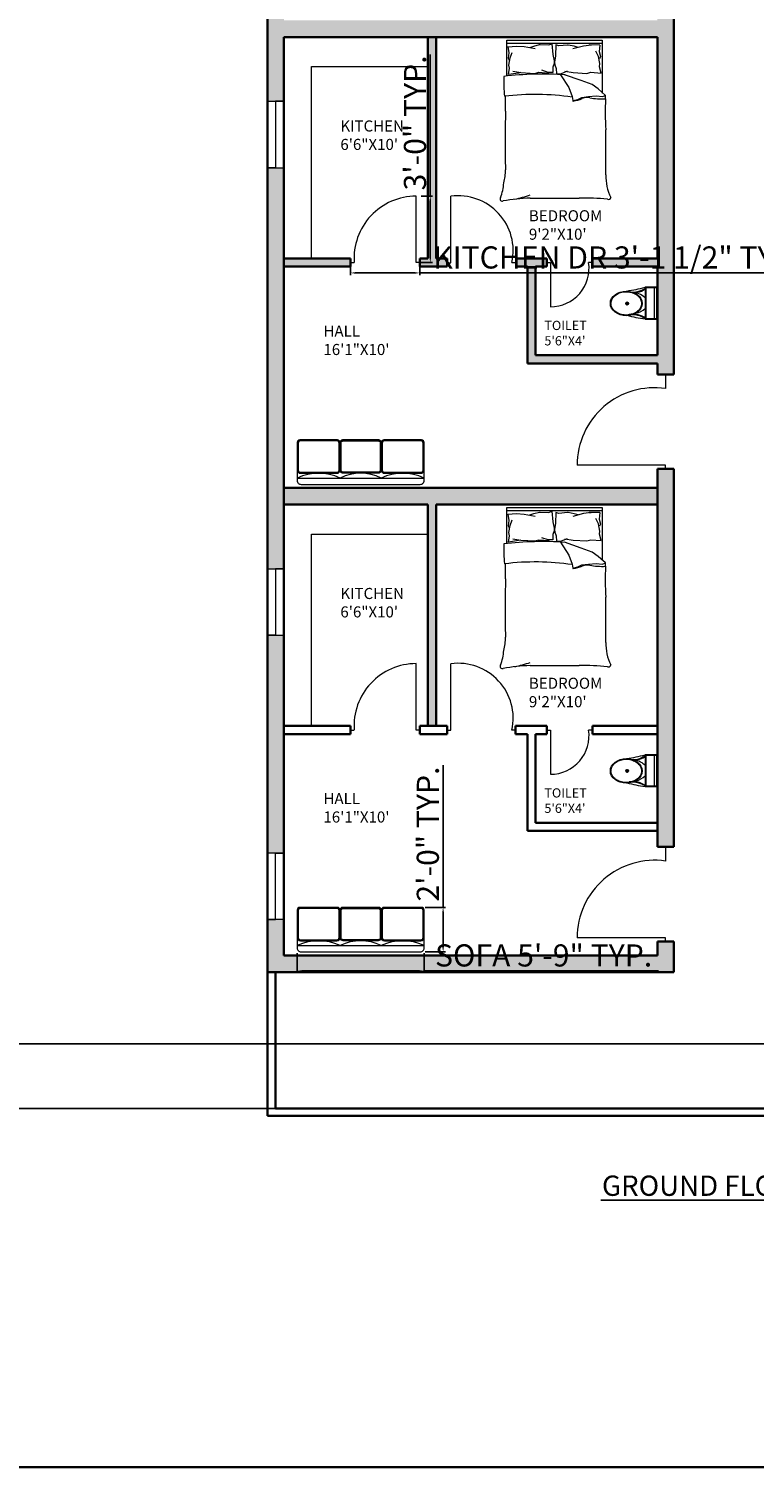
# Model space of a CAD drawing. Units: inches. Extents: x 1266 to 2869, y -408 to 3241.
# Tile 6 of 11: x 2023 to 2416, y 987 to 1767. Entities that reach past the tile are written whole.
import ezdxf

# ---------------------------------------------------------------- set-up
doc = ezdxf.new("R2010")
doc.units = ezdxf.units.IN
for name, color, linetype, lineweight in [('A-ANNO-DIMS', 2, 'Continuous', 18), ('A-ANNO-TITL', 7, 'Continuous', 25), ('A-ANNO-TTLB', 7, 'Continuous', 35), ('A-AREA-IDEN', 7, 'Continuous', 18), ('A-DOOR', 4, 'Continuous', 18), ('A-FLOR-CASE', 9, 'Continuous', 18), ('A-FLOR-FIXT', 9, 'Continuous', 18), ('A-FURN', 8, 'Continuous', 18), ('A-GLAZ', 4, 'Continuous', 18), ('A-WALL', 7, 'Continuous', 35), ('A-WALL-PATT', 251, 'Continuous', 13)]:
    doc.layers.add(name, color=color, linetype=linetype, lineweight=lineweight)
doc.styles.get("Standard").update_dxf_attribs({"font": 'arial.ttf'})
doc.dimstyles.new('ISO-25', dxfattribs={"dimtxt": 12, "dimasz": 2.5, "dimexe": 1.25, "dimexo": 0.625, "dimtad": 1, "dimdec": 0, "dimlunit": 3, "dimtxsty": 'Standard', "dimcen": 2.5, "dimadec": 0, "dimazin": 0, "dimtfac": 1, "dimtdec": 0, "dimtmove": 0, "dimatfit": 3, "dimfxl": 1, "dimarcsym": 0})

# ---------------------------------------------------------------- blocks, each defined once
blk = doc.blocks.new('A$C31115884')
for p, q in [((283, 498), (223, 498)), ((258, 466), (258, 523)), ((0, 200), (0, 0)), ((520, 200), (0, 200)), ((510, 54), (0, 54)), ((10, 190), (10, 10)), ((510, 190), (10, 190)), ((10, 10), (510, 10)), ((510, 10), (510, 190)), ((520, 0), (520, 200)), ((0, 0), (520, 0))]:
    blk.add_line(p, q)
blk.add_circle((256, 496), 23.6)
for centre, radius, start, end in [((2778, -205), 2807, 165.4549, 171.7133), ((3237, 905), 2807, 188.2867, 194.5451), ((-295, 403), 365, 324.2091, 9.3499), ((-295, 403), 375, 324.2091, 9.3499), ((384, 406), 293, 190.2774, 224.1564), ((139, 406), 293, 315.8436, 2.6563), ((806, 403), 375, 179.2036, 215.7909), ((806, 403), 365, 170.6501, 215.7909)]:
    blk.add_arc(centre, radius, start, end)
blk.add_ellipse((256, 510), major_axis=(0, -261), ratio=0.772727)
blk.add_open_spline([(256, 259), (263, 259), (270, 260), (288, 262), (299, 265), (320, 273), (330, 278), (350, 291), (360, 299), (378, 316), (386, 326), (402, 347), (409, 358), (421, 383), (427, 395), (436, 422), (440, 436), (445, 465), (447, 480), (448, 509), (448, 524), (445, 553), (443, 568), (436, 596), (432, 610), (422, 636), (416, 649), (402, 672), (395, 683), (379, 703), (370, 712), (351, 728), (341, 735), (321, 746), (310, 751), (289, 757), (278, 759), (256, 761), (245, 761), (223, 757), (212, 754), (191, 746), (181, 741), (161, 728), (151, 720), (133, 703), (125, 693), (110, 672), (103, 660), (90, 636), (85, 623), (76, 596), (72, 582), (67, 553), (66, 538), (64, 509), (65, 494), (68, 465), (70, 450), (77, 422), (81, 408), (91, 382), (97, 370), (111, 346), (118, 335), (135, 316), (144, 307), (162, 291), (172, 284), (193, 273), (203, 269), (225, 262), (236, 260), (250, 259), (253, 259), (256, 259)], degree=3, knots=[0, 0, 0, 0, 0.110105, 0.110105, 0.285049, 0.285049, 0.459994, 0.459994, 0.634938, 0.634938, 0.809882, 0.809882, 0.984827, 0.984827, 1.159771, 1.159771, 1.334715, 1.334715, 1.50966, 1.50966, 1.684604, 1.684604, 1.859549, 1.859549, 2.034493, 2.034493, 2.209437, 2.209437, 2.384382, 2.384382, 2.559326, 2.559326, 2.73427, 2.73427, 2.909215, 2.909215, 3.084159, 3.084159, 3.259103, 3.259103, 3.434048, 3.434048, 3.608992, 3.608992, 3.783936, 3.783936, 3.958881, 3.958881, 4.133825, 4.133825, 4.30877, 4.30877, 4.483714, 4.483714, 4.658658, 4.658658, 4.833603, 4.833603, 5.008547, 5.008547, 5.183491, 5.183491, 5.358436, 5.358436, 5.53338, 5.53338, 5.708324, 5.708324, 5.883269, 5.883269, 6.058213, 6.058213, 6.233158, 6.233158, 6.283185, 6.283185, 6.283185, 6.283185])
blk = doc.blocks.new('BED-DOUBLE')
for p, q in [((3.76, 67.77), (3.76, 87.35)), ((3.76, 87.35), (55.42, 87.35)), ((55.42, 87.35), (55.42, 58.59)), ((3.76, 85.69), (55.42, 85.69)), ((4.21, 83.74), (8.84, 84.1)), ((4.21, 83.77), (4.84, 80.33)), ((4.84, 80.33), (4.37, 77.51)), ((5.46, 77.67), (6.55, 80.64)), ((8.84, 84.1), (8.96, 84.08)), ((8.96, 84.08), (13.09, 83.77)), ((13.09, 83.77), (19.03, 82.67)), ((16.06, 83.3), (18.25, 84.08)), ((18.25, 84.08), (21.37, 84.86)), ((21.37, 84.86), (21.72, 84.86)), ((21.72, 84.86), (26.53, 84.7)), ((26.53, 84.7), (28.09, 85.33)), ((28.09, 85.33), (28.71, 79.55)), ((28.71, 79.55), (29.34, 76.11)), ((29.98, 78.85), (29.57, 75.38)), ((30.24, 84.66), (29.98, 78.85)), ((31.84, 84.13), (30.24, 84.66)), ((36.63, 84.59), (31.84, 84.13)), ((36.98, 84.61), (36.63, 84.59)), ((40.14, 84.02), (36.98, 84.61)), ((45.31, 84.03), (39.45, 82.57)), ((42.38, 83.38), (40.14, 84.02)), ((49.42, 84.6), (45.31, 84.03)), ((54.17, 84.59), (48.33, 84.69)), ((48.33, 84.69), (49.42, 84.6)), ((53.3, 78.43), (52.03, 81.32)), ((54.17, 74.56), (53.3, 78.43)), ((54.17, 84.59), (53.76, 81.12)), ((53.76, 81.12), (54.41, 78.34)), ((54.41, 78.34), (53.85, 77.21)), ((4.37, 77.51), (4.99, 76.42)), ((4.52, 68.61), (5.15, 72.04)), ((4.84, 73.76), (5.46, 77.67)), ((5.15, 72.04), (4.84, 73.76)), ((6.9, 70.46), (11.26, 69.74)), ((26.06, 69.77), (22.66, 70.95)), ((29.34, 74.7), (28.71, 72.67)), ((28.71, 72.67), (28.71, 69.77)), ((29.34, 76.11), (29.34, 74.7)), ((29.57, 75.38), (29.66, 73.97)), ((29.66, 73.97), (30.41, 71.98)), ((30.41, 71.98), (30.59, 69.09)), ((33.24, 69.26), (36.56, 70.64)), ((35.2, 70.46), (39.56, 69.74)), ((53.97, 72.83), (54.17, 74.56)), ((54.81, 69.44), (53.97, 72.83)), ((10.03, 69.39), (4.52, 68.61)), ((11.26, 69.74), (10.03, 69.39)), ((11.26, 69.74), (18.84, 69.27)), ((18.84, 69.27), (20.95, 69.87)), ((20.95, 69.87), (26.5, 69.44)), ((28.71, 69.77), (26.06, 69.77)), ((30.59, 69.09), (33.24, 69.26)), ((32.71, 68.56), (37.24, 61.54)), ((43.94, 65.39), (34.92, 68.56)), ((39.56, 69.74), (47.14, 69.27)), ((49.96, 63.21), (43.94, 65.39)), ((47.14, 69.27), (49.26, 69.87)), ((49.26, 69.87), (54.81, 69.44)), ((53.15, 60.87), (49.96, 63.21)), ((37.24, 61.54), (39.08, 56.69)), ((39.08, 56.69), (39.42, 54.51)), ((39.42, 54.51), (42.1, 55.18)), ((42.1, 55.18), (44.27, 56.19)), ((44.27, 56.19), (47.96, 56.69)), ((47.96, 56.69), (52.14, 57.02)), ((52.14, 57.02), (55.49, 56.69)), ((57.15, 57.36), (53.15, 60.87)), ((55.49, 56.69), (57.15, 57.36)), ((57.24, 55.47), (57.15, 57.36, 4.18)), ((16.28, 1.69), (42.89, 1.69))]:
    blk.add_line(p, q)
for centre, radius, start, end in [((92.06, 65.63), 90.06, 178.72178, 185.60397), ((23.09, -109.45), 178.34, 86.08655, 96.78213), ((19.19, -81.63), 139.47, 81.78449, 96.90062), ((-180.86, 53.65), 183.89, 358.4762, 1.00819), ((33.68, 85.75), 32.06, 280.66171, 289.88058), ((47.29, 49.44), 6.73, 78.6608, 113.73842), ((55.49, 94.55), 39.11, 259.87628, 272.56571), ((197.03, 48.09), 139.99, 176.97912, 183.83645), ((524.11, 32.64), 521.39, 178.22771, 181.71854), ((39.6, 54.45), 0.199, 160.24637, 271.13765), ((-4874.07, 14.03), 4931.49, 0.00217, 0.28689), ((-29.08, 17.61), 32.04, 346.06484, 358.91125), ((-23.41, 11.38), 25.47, 337.97508, 356.652), ((82.33, 13.12), 24.93, 177.47136, 206.46809), ((1.18, 1.17), 1.18, 146.17358, 293.47814), ((23.16, -129.76), 131.62, 92.99578, 99.40907), ((-18.62, 112.98), 115.08, 283.38322, 287.70533), ((44.49, -142.13), 143.82, 84.4998, 90.63509), ((58.82, 2.09), 1.19, 242.65876, 356.02002)]:
    blk.add_arc(centre, radius, start, end)
blk = doc.blocks.new('SOFA-3-SEAT-4')
for points in [[(0, 22.36), (0, 7.74, 0.414214), (1.72, 6.02), (21.5, 6.02, 0.414214), (23.22, 7.74), (23.22, 22.36, 0.414214), (21.5, 24.08), (1.72, 24.08, 0.414214)], [(0.52, 22.36), (0.52, 7.74, 0.414214), (1.72, 6.54), (21.5, 6.54, 0.414214), (22.7, 7.74), (22.7, 22.36, 0.414214), (21.5, 23.56), (1.72, 23.56, 0.414214)], [(45.57, 22.36), (45.57, 7.74, -0.414214), (43.85, 6.02), (24.94, 6.02, -0.414214), (23.22, 7.74), (23.22, 22.36, -0.414214), (24.94, 24.08), (43.85, 24.08, -0.414214)], [(45.06, 22.36), (45.06, 7.74, -0.414214), (43.85, 6.54), (24.94, 6.54, -0.414214), (23.73, 7.74), (23.73, 22.36, -0.414214), (24.94, 23.56), (43.85, 23.56, -0.414214)], [(45.57, 22.36), (45.57, 7.74, 0.414214), (47.29, 6.02), (67.07, 6.02, 0.414214), (68.79, 7.74), (68.79, 22.36, 0.414214), (67.07, 24.08), (47.29, 24.08, 0.414214)], [(46.09, 22.36), (46.09, 7.74, 0.414214), (47.29, 6.54), (67.07, 6.54, 0.414214), (68.27, 7.74), (68.27, 22.36, 0.414214), (67.07, 23.56), (47.29, 23.56, 0.414214)]]:
    blk.add_lwpolyline(points, format="xyb", close=True)
at = {"ltscale": 0.03}
blk.add_lwpolyline([(21.82, 24.08), (1.38, 24.08, 0.414214), (0, 22.7), (0, 2.06, 0.414214), (2.06, 0), (66.73, 0, 0.414214), (68.79, 2.06), (68.79, 22.7, 0.414214), (67.41, 24.08), (46.97, 24.08, 0.414214), (45.59, 22.7, -1), (45.56, 22.7, 0.414214), (44.18, 24.08), (24.61, 24.08, 0.414214), (23.23, 22.7, -1), (23.2, 22.7, 0.414214)], format="xyb", close=True, dxfattribs=at)
blk.add_lwpolyline([(0, 3.44), (68.79, 3.44)])
for centre, radius, start, end in [((11.61, -21.35), 27.38, 64.91063, 115.08937), ((34.4, -19.35), 25.38, 63.869, 116.131), ((57.18, -21.07), 27.12, 64.65382, 115.34618)]:
    blk.add_arc(centre, radius, start, end)
blk = doc.blocks.new('DOOR-KITCHEN-L')
for p, q in [((35.61, 0), (35.61, 36)), ((0, 0), (2, 0)), ((37.61, 0), (35.61, 0))]:
    blk.add_line(p, q)
blk.add_arc((35.61, 2.31), 33.69, 90, 183.92625)
blk = doc.blocks.new('DOOR-BEDROOM-L')
for p, q in [((2, 0), (2, 36)), ((0, 0), (2, 0)), ((37.12, 0.11), (35.12, 0.11))]:
    blk.add_line(p, q)
blk.add_arc((5.98, 6.45), 29.82, 347.72217, 97.67592)
blk = doc.blocks.new('DOOR-BATH-L')
for p, q in [((0, 24), (2, 24)), ((2, 24), (2, 0)), ((24.7, 24), (22.7, 24))]:
    blk.add_line(p, q)
blk.add_arc((2, 20.92), 20.92, 270, 8.45113)
blk = doc.blocks.new('DOOR-ENTRY-L')
for p, q in [((48, 51.27), (48, 45.59)), ((48, 45.59), (48, 43.59)), ((12, 2), (0, 2)), ((48, 2), (12, 2)), ((48, 0), (48, 2))]:
    blk.add_line(p, q)
blk.add_arc((42.02, 2), 42.02, 81.81164, 180)
blk = doc.blocks.new('WIN-PLAN-36')
for p, q in [((0, 36), (9, 36)), ((4.5, 36), (4.5, 0)), ((9, 36), (4.5, 36)), ((4.5, 0), (0, 0)), ((0, 0), (9, 0))]:
    blk.add_line(p, q)
blk = doc.blocks.new('COUNTER-KITCHEN-2')
for p, q in [((0, 0), (0, 103.95)), ((0, 103.95), (63, 103.95))]:
    blk.add_line(p, q)
blk = doc.blocks.new('*D43')
at = {"layer": 'A-ANNO-DIMS', "color": 0, "lineweight": -2, "transparency": 16777216}
for p, q in [((2197.56, 1639.47), (2197.56, 1633.21)), ((2235.18, 1639.47), (2235.18, 1633.21)), ((2200.06, 1634.46), (2232.68, 1634.46)), ((2235.18, 1634.46), (2446.61, 1634.46))]:
    blk.add_line(p, q, dxfattribs=at)
at = {"layer": 'A-ANNO-DIMS', "color": 0, "transparency": 16777216}
for points in [[(2200.06, 1634.87), (2200.06, 1634.04), (2197.56, 1634.46)], [(2232.68, 1634.87), (2232.68, 1634.04), (2235.18, 1634.46)]]:
    blk.add_solid(points, dxfattribs=at)
at = {"layer": 'Defpoints', "color": 0, "transparency": 16777216}
for p in [(2197.56, 1640.1), (2235.18, 1640.1), (2235.18, 1634.46)]:
    blk.add_point(p, dxfattribs=at)
at = {"layer": 'A-ANNO-DIMS', "color": 0, "transparency": 16777216, "insert": (2342.14, 1641.29), "char_height": 12, "attachment_point": 5}
blk.add_mtext('KITCHEN DR 3\'-1 1/2" TYP.', dxfattribs=at)
blk = doc.blocks.new('*D44')
at = {"layer": 'A-ANNO-DIMS', "color": 0, "lineweight": -2, "transparency": 16777216}
for p, q in [((2240.82, 1676.1), (2240.82, 1752.98)), ((2235.8, 1676.1), (2242.07, 1676.1)), ((2240.82, 1642.6), (2240.82, 1673.6)), ((2235.8, 1640.1), (2242.07, 1640.1))]:
    blk.add_line(p, q, dxfattribs=at)
at = {"layer": 'A-ANNO-DIMS', "color": 0, "transparency": 16777216}
for points in [[(2240.4, 1673.6), (2241.24, 1673.6), (2240.82, 1676.1)], [(2240.4, 1642.6), (2241.24, 1642.6), (2240.82, 1640.1)]]:
    blk.add_solid(points, dxfattribs=at)
at = {"layer": 'Defpoints', "color": 0, "transparency": 16777216}
for p in [(2235.18, 1676.1), (2240.82, 1676.1), (2235.18, 1640.1)]:
    blk.add_point(p, dxfattribs=at)
at = {"layer": 'A-ANNO-DIMS', "color": 0, "transparency": 16777216, "insert": (2234.06, 1715.79), "char_height": 12, "attachment_point": 5, "rotation": 90}
blk.add_mtext('3\'-0" TYP.', dxfattribs=at)
blk = doc.blocks.new('*D73')
at = {"layer": 'A-ANNO-DIMS', "color": 0, "lineweight": -2, "transparency": 16777216}
for p, q in [((2168.66, 1265.67), (2168.66, 1254.73)), ((2237.45, 1265.67), (2237.45, 1254.73)), ((2171.16, 1255.98), (2234.95, 1255.98)), ((2237.45, 1255.98), (2364.59, 1255.98))]:
    blk.add_line(p, q, dxfattribs=at)
at = {"layer": 'A-ANNO-DIMS', "color": 0, "transparency": 16777216}
for points in [[(2171.16, 1256.4), (2171.16, 1255.56), (2168.66, 1255.98)], [(2234.95, 1256.4), (2234.95, 1255.56), (2237.45, 1255.98)]]:
    blk.add_solid(points, dxfattribs=at)
at = {"layer": 'Defpoints', "color": 0, "transparency": 16777216}
for p in [(2168.66, 1266.3), (2237.45, 1266.3), (2237.45, 1255.98)]:
    blk.add_point(p, dxfattribs=at)
at = {"layer": 'A-ANNO-DIMS', "color": 0, "transparency": 16777216, "insert": (2302.27, 1262.81), "char_height": 12, "attachment_point": 5}
blk.add_mtext('SOFA 5\'-9" TYP.', dxfattribs=at)
blk = doc.blocks.new('*D74')
at = {"layer": 'A-ANNO-DIMS', "color": 0, "lineweight": -2, "transparency": 16777216}
for p, q in [((2247.77, 1290.38), (2247.77, 1367.48)), ((2238.07, 1290.38), (2249.02, 1290.38)), ((2247.77, 1268.8), (2247.77, 1287.88)), ((2238.07, 1266.3), (2249.02, 1266.3))]:
    blk.add_line(p, q, dxfattribs=at)
at = {"layer": 'A-ANNO-DIMS', "color": 0, "transparency": 16777216}
for points in [[(2247.35, 1287.88), (2248.18, 1287.88), (2247.77, 1290.38)], [(2247.35, 1268.8), (2248.18, 1268.8), (2247.77, 1266.3)]]:
    blk.add_solid(points, dxfattribs=at)
at = {"layer": 'Defpoints', "color": 0, "transparency": 16777216}
for p in [(2237.45, 1290.38), (2247.77, 1290.38), (2237.45, 1266.3)]:
    blk.add_point(p, dxfattribs=at)
at = {"layer": 'A-ANNO-DIMS', "color": 0, "transparency": 16777216, "insert": (2241.02, 1330.18), "char_height": 12, "attachment_point": 5, "rotation": 90}
blk.add_mtext('2\'-0" TYP.', dxfattribs=at)
blk = doc.blocks.new('*D87')
at = {"layer": 'A-ANNO-DIMS', "color": 0, "lineweight": -2, "transparency": 16777216}
for p, q in [((1969.26, 1216.35), (1969.26, 1261.52)), ((2453.69, 1216.35), (1968.01, 1216.35)), ((1969.26, 1183.9), (1969.26, 1213.85)), ((2453.69, 1181.4), (1968.01, 1181.4))]:
    blk.add_line(p, q, dxfattribs=at)
at = {"layer": 'A-ANNO-DIMS', "color": 0, "transparency": 16777216}
for points in [[(1968.84, 1213.85), (1969.68, 1213.85), (1969.26, 1216.35)], [(1968.84, 1183.9), (1969.68, 1183.9), (1969.26, 1181.4)]]:
    blk.add_solid(points, dxfattribs=at)
at = {"layer": 'Defpoints', "color": 0, "transparency": 16777216}
for p in [(1969.26, 1216.35), (2454.31, 1216.35), (2454.31, 1181.4)]:
    blk.add_point(p, dxfattribs=at)
at = {"layer": 'A-ANNO-DIMS', "color": 0, "transparency": 16777216, "insert": (1962.61, 1240.19), "char_height": 12, "attachment_point": 5, "rotation": 90}
blk.add_mtext('2\'-11"', dxfattribs=at)

msp = doc.modelspace()

# ---------------------------------------------------------------- hatches: boundary and pattern name
at = {"layer": 'A-WALL-PATT'}
h = msp.add_hatch(color=256, dxfattribs=at)
h.dxf.hatch_style = 1
h.paths.add_polyline_path([(2161.45, 2269.35), (2239.45, 2269.35), (2239.45, 2149.35), (2235.18, 2149.35), (2235.18, 2144.85), (2243.95, 2144.85), (2249.99, 2144.85), (2249.99, 2146.74), (2249.99, 2149.35), (2243.95, 2149.35), (2243.95, 2269.35), (2274.21, 2269.35), (2274.21, 2273.85), (2274.21, 2278.35), (2152.45, 2278.35), (2152.45, 2234.52), (2161.45, 2234.52)])
h.paths.add_polyline_path([(2550.01, 2278.35), (2424.95, 2278.35), (2372.95, 2278.35), (2334.21, 2278.35), (2334.21, 2269.35), (2363.95, 2269.35), (2363.95, 2149.35), (2328.7, 2149.35), (2328.7, 2144.85), (2363.95, 2144.85), (2363.95, 2133.61), (2372.95, 2133.61), (2372.95, 2269.35), (2424.95, 2269.35), (2424.95, 2234.52), (2433.95, 2234.52), (2433.95, 2269.35), (2511.95, 2269.35), (2511.95, 2149.35), (2504.09, 2149.35), (2504.09, 2144.85), (2520.49, 2144.85), (2520.49, 2149.35), (2516.45, 2149.35), (2516.45, 2269.35), (2550.01, 2269.35), (2550.01, 2273.85)])
h.paths.add_polyline_path([(2635.45, 2278.35), (2610.01, 2278.35), (2610.01, 2269.35), (2626.45, 2269.35), (2626.45, 2149.35), (2588.98, 2149.35), (2588.98, 2144.85), (2626.45, 2144.85), (2626.45, 2133.61), (2635.45, 2133.61)])
h.paths.add_polyline_path([(2560.45, 2144.85), (2565.84, 2144.85), (2565.84, 2149.35), (2552.33, 2149.35), (2552.33, 2144.85), (2555.95, 2144.85), (2555.95, 2092.35), (2626.45, 2092.35), (2626.45, 2086.89), (2626.45, 2024.85), (2610.01, 2024.85), (2610.01, 2015.85), (2626.45, 2015.85), (2626.45, 1895.85), (2589.21, 1895.85), (2589.21, 1891.35), (2626.45, 1891.35), (2626.45, 1880.11), (2635.45, 1880.11), (2635.45, 2086.89), (2635.45, 2109.61), (2626.45, 2109.61), (2626.45, 2096.85), (2560.45, 2096.85)])
h.paths.add_polyline_path([(2433.95, 2198.52), (2424.95, 2198.52), (2424.95, 2086.89), (2433.95, 2086.89), (2433.95, 2144.85), (2470.3, 2144.85), (2470.3, 2149.35), (2433.95, 2149.35)])
h.paths.add_polyline_path([(2372.95, 2109.61), (2363.95, 2109.61), (2363.95, 2096.85), (2297.95, 2096.85), (2297.95, 2144.85), (2304, 2144.85), (2304, 2149.35), (2293.45, 2149.35), (2287.11, 2149.35), (2287.11, 2144.85), (2293.45, 2144.85), (2293.45, 2092.35), (2363.95, 2092.35), (2363.95, 2086.89), (2372.95, 2086.89)], flags=17)
h.paths.add_polyline_path([(2161.45, 2144.85), (2197.56, 2144.85), (2197.56, 2149.35), (2161.45, 2149.35), (2161.45, 2198.52), (2152.45, 2198.52), (2152.45, 1981.02), (2161.45, 1981.02), (2161.45, 2015.85), (2363.95, 2015.85), (2363.95, 1895.85), (2326.89, 1895.85), (2326.89, 1891.35), (2363.95, 1891.35), (2363.95, 1880.11), (2372.95, 1880.11), (2372.95, 2035.62), (2363.95, 2035.62), (2363.95, 2024.85), (2161.45, 2024.85)])
h.paths.add_polyline_path([(2161.45, 1691.52), (2152.45, 1691.52), (2152.45, 1474.02), (2161.45, 1474.02)])
h.paths.add_polyline_path([(2194.79, 1895.85), (2161.45, 1895.85), (2161.45, 1945.02), (2152.45, 1945.02), (2152.45, 1727.52), (2161.45, 1727.52), (2161.45, 1762.35), (2363.95, 1762.35), (2363.95, 1642.35), (2328.7, 1642.35), (2328.7, 1637.85), (2363.95, 1637.85), (2363.95, 1589.85), (2297.95, 1589.85), (2297.95, 1637.85), (2303.95, 1637.85), (2303.95, 1642.35), (2287.64, 1642.35), (2287.64, 1637.85), (2293.45, 1637.85), (2293.45, 1585.35), (2363.95, 1585.35), (2363.95, 1579.45), (2372.95, 1579.45), (2372.95, 1779.84), (2363.95, 1779.84), (2363.95, 1771.35), (2161.45, 1771.35), (2161.45, 1891.35), (2194.79, 1891.35)])
h.paths.add_polyline_path([(2243.95, 2015.85), (2239.45, 2015.85), (2239.45, 1895.85), (2232.4, 1895.85), (2232.4, 1891.35), (2247.22, 1891.35), (2247.22, 1895.85), (2243.95, 1895.85)], flags=17)
h.paths.add_polyline_path([(2302.19, 1895.85), (2284.34, 1895.85), (2284.34, 1891.35), (2293.45, 1891.35), (2293.45, 1838.85), (2363.95, 1838.85), (2363.95, 1831.11), (2372.95, 1831.11), (2372.95, 1856.11), (2363.95, 1856.11), (2363.95, 1843.35), (2297.95, 1843.35), (2297.95, 1891.35), (2302.19, 1891.35)], flags=17)
h.paths.add_polyline_path([(2243.95, 1762.35), (2239.45, 1762.35), (2239.45, 1642.35), (2235.18, 1642.35), (2235.18, 1637.85), (2249.99, 1637.85), (2249.99, 1642.35), (2243.95, 1642.35)], flags=17)
h.paths.add_polyline_path([(2197.56, 1642.35), (2161.45, 1642.35), (2161.45, 1637.85), (2197.56, 1637.85)], flags=17)
h.paths.add_polyline_path([(2363.95, 1517.85), (2161.45, 1517.85), (2161.45, 1508.85), (2239.45, 1508.85), (2239.45, 1388.85), (2243.95, 1388.85), (2243.95, 1508.85), (2363.95, 1508.85)])
h.paths.add_polyline_path([(2372.95, 1528.18), (2363.95, 1528.18), (2363.95, 1323.21), (2372.95, 1323.21)])
h.paths.add_polyline_path([(2372.95, 1271.94), (2363.95, 1271.94), (2363.95, 1264.35), (2161.45, 1264.35), (2161.45, 1283.77), (2156.95, 1283.77), (2152.45, 1283.77), (2152.45, 1255.35), (2156.95, 1255.35), (2372.95, 1255.35)])
h.paths.add_polyline_path([(2161.45, 1438.02), (2152.45, 1438.02), (2152.45, 1319.77), (2161.45, 1319.77)])
h.paths.add_polyline_path([(2550.01, 1513.35), (2550.01, 1517.85), (2433.95, 1517.85), (2433.95, 1528.62), (2424.95, 1528.62), (2424.95, 1474.02), (2433.95, 1474.02), (2433.95, 1508.85), (2511.95, 1508.85), (2511.95, 1388.85), (2504.09, 1388.85), (2504.09, 1384.35), (2520.49, 1384.35), (2520.49, 1388.85), (2516.45, 1388.85), (2516.45, 1508.85), (2550.01, 1508.85)])
h.paths.add_polyline_path([(2635.45, 1602.61), (2626.45, 1602.61), (2626.45, 1517.85), (2610.01, 1517.85), (2610.01, 1508.85), (2626.45, 1508.85), (2626.45, 1388.85), (2588.98, 1388.85), (2588.98, 1384.35), (2626.45, 1384.35), (2626.45, 1373.11), (2635.45, 1373.11)])
h.paths.add_polyline_path([(2635.45, 1349.11), (2626.45, 1349.11), (2626.45, 1336.35), (2560.45, 1336.35), (2560.45, 1384.35), (2565.84, 1384.35), (2565.84, 1388.85), (2552.33, 1388.85), (2552.33, 1384.35), (2555.95, 1384.35), (2555.95, 1331.85), (2626.45, 1331.85), (2626.45, 1315.59), (2635.45, 1315.59)])
h.paths.add_polyline_path([(2635.45, 1279.59), (2630.95, 1279.59), (2626.45, 1279.59), (2626.45, 1264.35), (2433.95, 1264.35), (2433.95, 1275.12), (2424.95, 1275.12), (2424.95, 1255.35), (2635.45, 1255.35)])
h.paths.add_polyline_path([(2433.95, 1438.02), (2424.95, 1438.02), (2424.95, 1326.39), (2433.95, 1326.39)])
h.paths.add_polyline_path([(2470.3, 1388.85), (2433.95, 1388.85), (2433.95, 1384.35), (2470.3, 1384.35)], flags=0)

# ---------------------------------------------------------------- linework, layer by layer
at = {"layer": 'A-ANNO-TITL'}
msp.add_line((2333.33, 1131.68), (2505.49, 1131.68), dxfattribs=at)
at = {"layer": 'A-ANNO-TTLB'}
msp.add_lwpolyline([(1266.23, 3241.34), (2868.62, 3241.34), (2868.62, 986.84), (1266.23, 986.84)], close=True, dxfattribs=at)
at = {"layer": 'A-DOOR'}
for p, q in [((2251.99, 1639.99), (2251.99, 1675.99)), ((2249.99, 1639.99), (2251.99, 1639.99)), ((2285.11, 1640.1), (2285.64, 1640.1)), ((2285.64, 1640.1), (2287.64, 1640.1))]:
    msp.add_line(p, q, dxfattribs=at)
msp.add_arc((2255.97, 1646.44), 29.82, 347.72217, 97.67592, dxfattribs=at)
at = {"layer": 'A-WALL'}
for p, q in [((2152.45, 2278.35), (2152.45, 1255.35)), ((2372.95, 1779.84), (2372.95, 1579.45)), ((2161.45, 1762.35), (2161.45, 1264.35)), ((2161.45, 1762.35), (2363.95, 1762.35)), ((2239.45, 1762.35), (2239.45, 1642.35)), ((2239.45, 1762.35), (2239.45, 1642.35)), ((2243.95, 1762.35), (2243.95, 1642.35)), ((2243.95, 1762.35), (2243.95, 1642.35)), ((2363.95, 1762.35), (2363.95, 1642.35)), ((2161.45, 1642.35), (2197.56, 1642.35)), ((2197.56, 1640.1), (2197.56, 1642.35)), ((2197.56, 1642.35), (2197.56, 1637.85)), ((2235.18, 1642.35), (2239.45, 1642.35)), ((2235.18, 1640.1), (2235.18, 1642.35)), ((2235.18, 1642.35), (2235.18, 1637.85)), ((2243.95, 1642.35), (2249.99, 1642.35)), ((2249.99, 1639.99), (2249.99, 1642.35)), ((2249.99, 1642.35), (2249.99, 1637.85)), ((2287.64, 1642.35), (2303.95, 1642.35)), ((2287.64, 1640.1), (2287.64, 1642.35)), ((2287.64, 1642.35), (2287.64, 1637.85)), ((2304, 1640.1), (2303.95, 1642.35)), ((2303.95, 1642.35), (2303.95, 1637.85)), ((2328.7, 1642.35), (2363.95, 1642.35)), ((2328.7, 1640.1), (2328.7, 1642.35)), ((2328.7, 1642.35), (2328.7, 1637.85)), ((2161.45, 1637.85), (2197.56, 1637.85)), ((2235.18, 1637.85), (2249.99, 1637.85)), ((2287.64, 1637.85), (2293.45, 1637.85)), ((2293.45, 1637.85), (2293.45, 1585.35)), ((2297.95, 1637.85), (2297.95, 1589.85)), ((2297.95, 1637.85), (2303.95, 1637.85)), ((2328.7, 1637.85), (2363.95, 1637.85)), ((2363.95, 1637.85), (2363.95, 1589.85)), ((2293.45, 1585.35), (2363.95, 1585.35)), ((2297.95, 1589.85), (2363.95, 1589.85)), ((2363.95, 1585.35), (2363.95, 1579.45)), ((2368.45, 1579.45), (2363.95, 1579.45)), ((2363.95, 1579.45), (2372.95, 1579.45)), ((2363.95, 1528.18), (2363.95, 1323.21)), ((2368.45, 1528.18), (2363.95, 1528.18)), ((2363.95, 1528.18), (2372.95, 1528.18)), ((2372.95, 1528.18), (2372.95, 1323.21)), ((2161.45, 1517.85), (2363.95, 1517.85)), ((2161.45, 1508.85), (2239.45, 1508.85)), ((2239.45, 1508.85), (2239.45, 1388.85)), ((2243.95, 1508.85), (2243.95, 1388.85)), ((2243.95, 1508.85), (2363.95, 1508.85)), ((2161.45, 1388.85), (2197.56, 1388.85)), ((2197.56, 1386.6), (2197.56, 1388.85)), ((2197.56, 1388.85), (2197.56, 1384.35)), ((2235.18, 1388.85), (2249.99, 1388.85)), ((2235.18, 1386.6), (2235.18, 1388.85)), ((2235.18, 1388.85), (2235.18, 1384.35)), ((2249.99, 1386.49), (2249.99, 1388.85)), ((2249.99, 1388.85), (2249.99, 1384.35)), ((2287.11, 1388.85), (2304, 1388.85)), ((2287.11, 1386.6), (2287.11, 1388.85)), ((2287.11, 1388.85), (2287.11, 1384.35)), ((2304, 1386.6), (2304, 1388.85)), ((2304, 1388.85), (2304, 1384.35)), ((2328.7, 1388.85), (2363.95, 1388.85)), ((2328.7, 1386.6), (2328.7, 1388.85)), ((2328.7, 1388.85), (2328.7, 1384.35)), ((2161.45, 1384.35), (2197.56, 1384.35)), ((2235.18, 1384.35), (2249.99, 1384.35)), ((2287.11, 1384.35), (2293.45, 1384.35)), ((2293.45, 1384.35), (2293.45, 1331.85)), ((2297.95, 1384.35), (2297.95, 1336.35)), ((2297.95, 1384.35), (2304, 1384.35)), ((2304, 1384.35), (2304, 1384.35)), ((2328.7, 1384.35), (2363.95, 1384.35)), ((2297.95, 1336.35), (2363.95, 1336.35)), ((2293.45, 1331.85), (2363.95, 1331.85)), ((2368.45, 1323.21), (2363.95, 1323.21)), ((2363.95, 1323.21), (2372.95, 1323.21)), ((2363.95, 1271.94), (2363.95, 1264.35)), ((2368.45, 1271.94), (2363.95, 1271.94)), ((2363.95, 1271.94), (2372.95, 1271.94)), ((2372.95, 1271.94), (2372.95, 1255.35)), ((2161.45, 1264.35), (2363.95, 1264.35)), ((2152.45, 1255.35), (2372.95, 1255.35)), ((2152.45, 1255.35), (2152.45, 1177.35)), ((2152.45, 1255.35), (2156.95, 1255.35)), ((2156.95, 1255.35), (2156.95, 1181.4)), ((2156.95, 1181.4), (2626.45, 1181.4)), ((2152.45, 1177.35), (2424.95, 1177.35))]:
    msp.add_line(p, q, dxfattribs=at)

# ---------------------------------------------------------------- block references
at = {"layer": 'A-DOOR'}
for name, p in [('DOOR-KITCHEN-L', (2197.56, 1640.1)), ('DOOR-BATH-L', (2304, 1616.1)), ('DOOR-ENTRY-L', (2320.45, 1528.18)), ('DOOR-KITCHEN-L', (2197.56, 1386.6)), ('DOOR-BEDROOM-L', (2249.99, 1386.49)), ('DOOR-BATH-L', (2304, 1362.6)), ('DOOR-ENTRY-L', (2320.45, 1271.94))]:
    msp.add_blockref(name, p, dxfattribs=at)
at = {"layer": 'A-FLOR-CASE'}
for p in [(2176.45, 1642.35), (2176.45, 1388.85)]:
    msp.add_blockref('COUNTER-KITCHEN-2', p, dxfattribs=at)
at = {"layer": 'A-FLOR-FIXT', "xscale": 0.0330640103915726, "yscale": 0.0330640103915726, "zscale": 0.0330640103915726, "rotation": 89.99999999999996}
for p in [(2363.95, 1609.46), (2363.95, 1355.96)]:
    msp.add_blockref('A$C31115884', p, dxfattribs=at)
at = {"layer": 'A-FURN'}
for name, p in [('BED-DOUBLE', (2278.65, 1673.39)), ('SOFA-3-SEAT-4', (2168.66, 1519.8)), ('BED-DOUBLE', (2278.65, 1419.89)), ('SOFA-3-SEAT-4', (2168.66, 1266.3))]:
    msp.add_blockref(name, p, dxfattribs=at)
at = {"layer": 'A-GLAZ'}
for p in [(2152.45, 1691.52), (2152.45, 1438.02)]:
    msp.add_blockref('WIN-PLAN-36', p, dxfattribs=at)
at = {"layer": 'A-GLAZ', "rotation": 180}
msp.add_blockref('WIN-PLAN-36', (2161.45, 1319.77), dxfattribs=at)

# ---------------------------------------------------------------- texts
at = {"layer": 'A-ANNO-TITL', "insert": (2333.93, 1145), "char_height": 11, "attachment_point": 1}
msp.add_mtext_dynamic_manual_height_columns('GROUND FLOOR PLAN', width=423.8424, gutter_width=12.5, heights=[0], dxfattribs=at)
at = {"layer": 'A-AREA-IDEN', "attachment_point": 1}
for s, width, insert, char_height in [('KITCHEN\\P6\'6"X10\'', 112.1355, (2192.04, 1717.14), 6), ('BEDROOM\\P9\'2"X10\'', 62.026, (2294.3, 1668.46), 6), ('TOILET\\P5\'6"X4\'', 46.3569, (2302.69, 1608.49), 5), ('HALL\\P16\'1"X10\'', 100.9767, (2182.86, 1605.93), 6), ('KITCHEN\\P6\'6"X10\'', 112.1355, (2192.04, 1463.64), 6), ('BEDROOM\\P9\'2"X10\'', 62.026, (2294.3, 1414.96), 6), ('HALL\\P16\'1"X10\'', 100.9767, (2182.86, 1352.43), 6), ('TOILET\\P5\'6"X4\'', 46.3569, (2302.69, 1354.99), 5)]:
    msp.add_mtext_dynamic_manual_height_columns(s, width=width, gutter_width=12.5, heights=[0], dxfattribs=dict(at, insert=insert, char_height=char_height))

# ---------------------------------------------------------------- dimensions: what is measured, and where the dimension line sits
at = {"layer": 'A-ANNO-DIMS'}
for base, p1, p2, picture, middle in [((2240.82, 1676.1), (2235.18, 1640.1), (2235.18, 1676.1), '*D44', (2234.06, 1715.79)), ((2247.77, 1290.38), (2237.45, 1266.3), (2237.45, 1290.38), '*D74', (2241.02, 1330.18))]:
    dim = msp.add_linear_dim(base=base, p1=p1, p2=p2, angle=90, text='<> TYP.', dimstyle='ISO-25', override={"dimdec": 1, "dimlfac": 1, "dimrnd": 0, "dimzin": 1, "dimdsep": 46, "dimlunit": 4, "dimfrac": 2}, dxfattribs=at)
    dim.commit()
    dim.dimension.update_dxf_attribs({"geometry": picture, "text_midpoint": middle})
for base, p1, p2, text, picture, middle in [((2235.18, 1634.46), (2197.56, 1640.1), (2235.18, 1640.1), 'KITCHEN DR <> TYP.', '*D43', (2342.14, 1641.29)), ((2237.45, 1255.98), (2168.66, 1266.3), (2237.45, 1266.3), 'SOFA <> TYP.', '*D73', (2302.27, 1262.81))]:
    dim = msp.add_linear_dim(base=base, p1=p1, p2=p2, text=text, dimstyle='ISO-25', override={"dimdec": 1, "dimlfac": 1, "dimrnd": 0, "dimzin": 1, "dimdsep": 46, "dimlunit": 4, "dimfrac": 2}, dxfattribs=at)
    dim.commit()
    dim.dimension.update_dxf_attribs({"geometry": picture, "text_midpoint": middle})
dim = msp.add_linear_dim(base=(1969.2585, 1216.3471), p1=(2454.3125, 1181.4021), p2=(2454.3125, 1216.3471), angle=90, dimstyle='ISO-25', override={"dimdec": 1, "dimlfac": 1, "dimrnd": 0, "dimzin": 1, "dimdsep": 46, "dimlunit": 4, "dimfrac": 2}, dxfattribs=at)
dim.commit()
dim.dimension.update_dxf_attribs({"geometry": '*D87', "text_midpoint": (1962.609, 1240.1856)})

doc.saveas('drawing.dxf')
